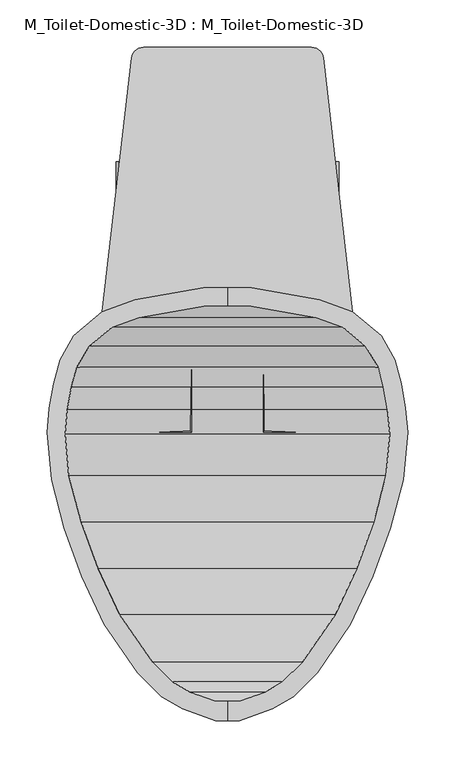
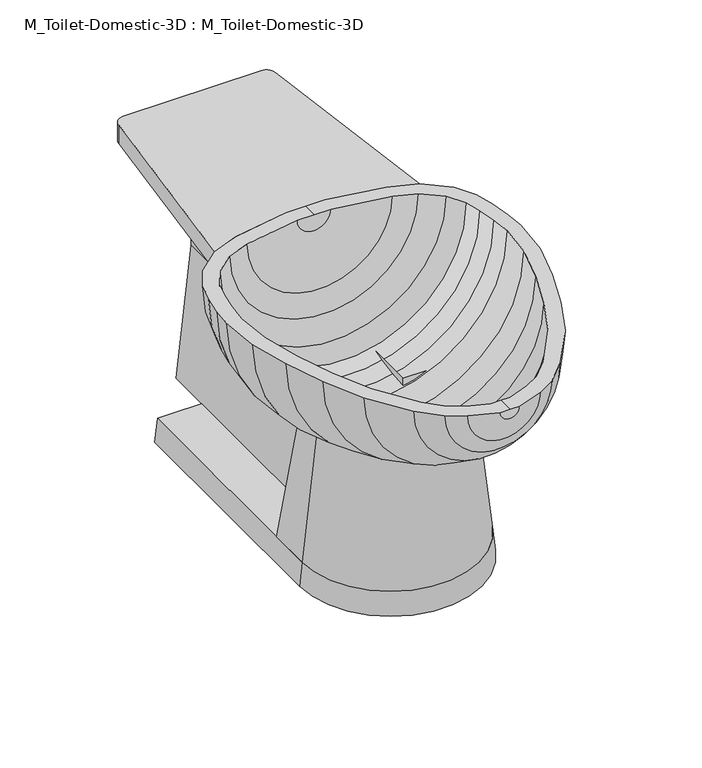
"""IFC4 building model written with IfcOpenShell, lengths in millimetres: flow terminal geometry, M_Toilet-Domestic-3D : M_Toilet-Domestic-3D."""

from ifc_helpers import new_model, si_unit, point, frame, frame_2d, origin, place, context, project, spatial, polyline, circle_curve, trimmed, segment, composite_curve, outline, extrude, source, transform, mapped, element, save
from ifc_brep_helpers import plane_surface, revolved_surface, advanced_brep


def m_toilet_domestic_3d_m_toilet_domestic_3d_ba6479b0(model_context):
    return source(origin(), model_context, "Body", "SolidModel", [
        advanced_brep(
        [(-25.4, 152.4, 361.95), (-97.4252791, 139.7, 361.95), (-132.3182423, 127.0, 361.95), (-162.5887836, 101.6, 361.95), (-176.9845865, 76.2, 361.95), (-183.790496, 50.8, 361.95), (-188.2862441, 25.3033453, 361.95), (-190.5, 0.0, 361.95), (-186.0724883, -50.6066907, 361.95), (-172.4088722, -101.6, 361.95), (-153.9191843, -152.4, 361.95), (-130.2307553, -203.2, 361.95), (-94.9900085, -254.0, 361.95), (-69.5900085, -279.4, 361.95), (-47.5929632, -292.1, 361.95), (-12.7, -304.8, 361.95), (0.0, -304.8, 361.95), (0.0, -284.592034, 361.95), (-12.5224565, -284.592034, 361.95), (-39.5113323, -274.7688865, 361.95), (-58.4178985, -263.8531754, 361.95), (-79.2146703, -243.0564036, 361.95), (-114.0255101, -192.8761202, 361.95), (-136.654021, -144.3491221, 361.95), (-154.575847, -95.1093097, 361.95), (-167.7238545, -46.0402777, 361.95), (-171.5645445, -2.1409906, 361.95), (-169.3087351, 23.6430284, 361.95), (-165.101298, 47.5045901, 361.95), (-159.5484355, 68.2281551, 361.95), (-146.1085923, 90.5605136, 361.95), (-121.9980886, 110.7916284, 361.95), (-94.1172813, 120.9394123, 361.95), (-22.0920022, 133.6394123, 361.95), (0.0, 133.6394123, 361.95), (0.0, 152.4, 361.95), (25.4, 152.4, 361.95), (22.0920022, 133.6394123, 361.95), (94.1172813, 120.9394123, 361.95), (121.9980886, 110.7916284, 361.95), (146.1085923, 90.5605136, 361.95), (159.5484355, 68.2281551, 361.95), (165.101298, 47.5045901, 361.95), (169.3087351, 23.6430284, 361.95), (171.5645445, -2.1409906, 361.95), (167.7238545, -46.0402777, 361.95), (154.575847, -95.1093097, 361.95), (136.654021, -144.3491221, 361.95), (114.0255101, -192.8761202, 361.95), (79.2146703, -243.0564036, 361.95), (58.4178985, -263.8531754, 361.95), (39.5113323, -274.7688865, 361.95), (12.5224565, -284.592034, 361.95), (12.7, -304.8, 361.95), (47.5929632, -292.1, 361.95), (69.5900085, -279.4, 361.95), (94.9900085, -254.0, 361.95), (130.2307553, -203.2, 361.95), (153.9191843, -152.4, 361.95), (172.4088722, -101.6, 361.95), (186.0724883, -50.6066907, 361.95), (190.5, 0.0, 361.95), (188.2862441, 25.3033453, 361.95), (183.790496, 50.8, 361.95), (176.9845865, 76.2, 361.95), (162.5887836, 101.6, 361.95), (132.3182423, 127.0, 361.95), (97.4252791, 139.7, 361.95)],
        [
            (0, 1),
            (1, 2),
            (2, 3),
            (3, 4),
            (4, 5),
            (5, 6),
            (6, 7),
            (7, 8),
            (8, 9),
            (9, 10),
            (10, 11),
            (11, 12),
            (12, 13),
            (13, 14),
            (14, 15),
            (15, 16),
            (16, 17),
            (17, 18),
            (18, 19),
            (19, 20),
            (20, 21),
            (21, 22),
            (22, 23),
            (23, 24),
            (24, 25),
            (25, 26),
            (26, 27),
            (27, 28),
            (28, 29),
            (29, 30),
            (30, 31),
            (31, 32),
            (32, 33),
            (33, 34),
            (34, 35),
            (35, 0),
            (36, 35),
            (34, 37),
            (37, 38),
            (38, 39),
            (39, 40),
            (40, 41),
            (41, 42),
            (42, 43),
            (43, 44),
            (44, 45),
            (45, 46),
            (46, 47),
            (47, 48),
            (48, 49),
            (49, 50),
            (50, 51),
            (51, 52),
            (52, 17),
            (16, 53),
            (53, 54),
            (54, 55),
            (55, 56),
            (56, 57),
            (57, 58),
            (58, 59),
            (59, 60),
            (60, 61),
            (61, 62),
            (62, 63),
            (63, 64),
            (64, 65),
            (65, 66),
            (66, 67),
            (67, 36),
            (67, 1, circle_curve(frame((0.0, 139.7, 361.95), z_axis=(0.0, 1.0, 0.0), x_axis=(-1.0, 0.0, 0.0)), 97.4252791)),
            (0, 36, circle_curve(frame((0.0, 152.4, 361.95), z_axis=(0.0, -1.0, 0.0), x_axis=(-1.0, 0.0, 0.0)), 25.4)),
            (66, 2, circle_curve(frame((0.0, 127.0, 361.95), z_axis=(0.0, 1.0, 0.0), x_axis=(-1.0, 0.0, 0.0)), 132.3182423)),
            (65, 3, circle_curve(frame((0.0, 101.6, 361.95), z_axis=(0.0, 1.0, 0.0), x_axis=(-1.0, 0.0, 0.0)), 162.5887836)),
            (64, 4, circle_curve(frame((0.0, 76.2, 361.95), z_axis=(0.0, 1.0, 0.0), x_axis=(-1.0, 0.0, 0.0)), 176.9845865)),
            (63, 5, circle_curve(frame((0.0, 50.8, 361.95), z_axis=(0.0, 1.0, 0.0), x_axis=(-1.0, 0.0, 0.0)), 183.790496)),
            (62, 6, circle_curve(frame((0.0, 25.3033453, 361.95), z_axis=(0.0, 1.0, 0.0), x_axis=(-1.0, 0.0, 0.0)), 188.2862441)),
            (61, 7, circle_curve(frame((0.0, 0.0, 361.95), z_axis=(0.0, 1.0, 0.0), x_axis=(-1.0, 0.0, 0.0)), 190.5)),
            (60, 8, circle_curve(frame((0.0, -50.6066907, 361.95), z_axis=(0.0, 1.0, 0.0), x_axis=(-1.0, 0.0, 0.0)), 186.0724883)),
            (59, 9, circle_curve(frame((0.0, -101.6, 361.95), z_axis=(0.0, 1.0, 0.0), x_axis=(-1.0, 0.0, 0.0)), 172.4088722)),
            (58, 10, circle_curve(frame((0.0, -152.4, 361.95), z_axis=(0.0, 1.0, 0.0), x_axis=(-1.0, 0.0, 0.0)), 153.9191843)),
            (57, 11, circle_curve(frame((0.0, -203.2, 361.95), z_axis=(0.0, 1.0, 0.0), x_axis=(-1.0, 0.0, 0.0)), 130.2307553)),
            (56, 12, circle_curve(frame((0.0, -254.0, 361.95), z_axis=(0.0, 1.0, 0.0), x_axis=(-1.0, 0.0, 0.0)), 94.9900085)),
            (55, 13, circle_curve(frame((0.0, -279.4, 361.95), z_axis=(0.0, 1.0, 0.0), x_axis=(-1.0, 0.0, 0.0)), 69.5900085)),
            (54, 14, circle_curve(frame((0.0, -292.1, 361.95), z_axis=(0.0, 1.0, 0.0), x_axis=(-1.0, 0.0, 0.0)), 47.5929632)),
            (53, 15, circle_curve(frame((0.0, -304.8, 361.95), z_axis=(0.0, 1.0, 0.0), x_axis=(-1.0, 0.0, 0.0)), 12.7)),
            (52, 18, circle_curve(frame((0.0, -284.592034, 361.95), z_axis=(0.0, 1.0, 0.0), x_axis=(-1.0, 0.0, 0.0)), 12.5224565)),
            (51, 19, circle_curve(frame((0.0, -274.7688865, 361.95), z_axis=(0.0, 1.0, 0.0), x_axis=(-1.0, 0.0, 0.0)), 39.5113323)),
            (50, 20, circle_curve(frame((0.0, -263.8531754, 361.95), z_axis=(0.0, 1.0, 0.0), x_axis=(-1.0, 0.0, 0.0)), 58.4178985)),
            (49, 21, circle_curve(frame((0.0, -243.0564036, 361.95), z_axis=(0.0, 1.0, 0.0), x_axis=(-1.0, 0.0, 0.0)), 79.2146703)),
            (48, 22, circle_curve(frame((0.0, -192.8761202, 361.95), z_axis=(0.0, 1.0, 0.0), x_axis=(-1.0, 0.0, 0.0)), 114.0255101)),
            (47, 23, circle_curve(frame((0.0, -144.3491221, 361.95), z_axis=(0.0, 1.0, 0.0), x_axis=(-1.0, 0.0, 0.0)), 136.654021)),
            (46, 24, circle_curve(frame((0.0, -95.1093097, 361.95), z_axis=(0.0, 1.0, 0.0), x_axis=(-1.0, 0.0, 0.0)), 154.575847)),
            (45, 25, circle_curve(frame((0.0, -46.0402777, 361.95), z_axis=(0.0, 1.0, 0.0), x_axis=(-1.0, 0.0, 0.0)), 167.7238545)),
            (44, 26, circle_curve(frame((0.0, -2.1409906, 361.95), z_axis=(0.0, 1.0, 0.0), x_axis=(-1.0, 0.0, 0.0)), 171.5645445)),
            (43, 27, circle_curve(frame((0.0, 23.6430284, 361.95), z_axis=(0.0, 1.0, 0.0), x_axis=(-1.0, 0.0, 0.0)), 169.3087351)),
            (42, 28, circle_curve(frame((0.0, 47.5045901, 361.95), z_axis=(0.0, 1.0, 0.0), x_axis=(-1.0, 0.0, 0.0)), 165.101298)),
            (41, 29, circle_curve(frame((0.0, 68.2281551, 361.95), z_axis=(0.0, 1.0, 0.0), x_axis=(-1.0, 0.0, 0.0)), 159.5484355)),
            (40, 30, circle_curve(frame((0.0, 90.5605136, 361.95), z_axis=(0.0, 1.0, 0.0), x_axis=(-1.0, 0.0, 0.0)), 146.1085923)),
            (39, 31, circle_curve(frame((0.0, 110.7916284, 361.95), z_axis=(0.0, 1.0, 0.0), x_axis=(-1.0, 0.0, 0.0)), 121.9980886)),
            (38, 32, circle_curve(frame((0.0, 120.9394123, 361.95), z_axis=(0.0, 1.0, 0.0), x_axis=(-1.0, 0.0, 0.0)), 94.1172813)),
            (37, 33, circle_curve(frame((0.0, 133.6394123, 361.95), z_axis=(0.0, 1.0, 0.0), x_axis=(-1.0, 0.0, 0.0)), 22.0920022)),
        ],
        [
            plane_surface(frame((0.0, 175.1599017, 361.95), z_axis=(0.0, 0.0, 1.0), x_axis=(-1.0, 0.0, 0.0))),
            plane_surface(frame((0.0, 175.1599017, 361.95), z_axis=(0.0, 0.0, 1.0), x_axis=(1.0, 0.0, 0.0))),
            revolved_surface(polyline([(-25.4, 152.4, 361.95), (-97.4252791, 139.7, 361.95)]), (0.0, 175.1599017, 361.95), (0.0, -1.0, 0.0)),
            revolved_surface(polyline([(-97.4252791, 139.7, 361.95), (-132.3182423, 127.0, 361.95)]), (0.0, 175.1599017, 361.95), (0.0, -1.0, 0.0)),
            revolved_surface(polyline([(-132.3182423, 127.0, 361.95), (-162.5887836, 101.6, 361.95)]), (0.0, 175.1599017, 361.95), (0.0, -1.0, 0.0)),
            revolved_surface(polyline([(-162.5887836, 101.6, 361.95), (-176.9845865, 76.2, 361.95)]), (0.0, 175.1599017, 361.95), (0.0, -1.0, 0.0)),
            revolved_surface(polyline([(-176.9845865, 76.2, 361.95), (-183.790496, 50.8, 361.95)]), (0.0, 175.1599017, 361.95), (0.0, -1.0, 0.0)),
            revolved_surface(polyline([(-183.790496, 50.8, 361.95), (-188.2862441, 25.3033453, 361.95)]), (0.0, 175.1599017, 361.95), (0.0, -1.0, 0.0)),
            revolved_surface(polyline([(-188.2862441, 25.3033453, 361.95), (-190.5, 0.0, 361.95)]), (0.0, 175.1599017, 361.95), (0.0, -1.0, 0.0)),
            revolved_surface(polyline([(-190.5, 0.0, 361.95), (-186.0724883, -50.6066907, 361.95)]), (0.0, 175.1599017, 361.95), (0.0, -1.0, 0.0)),
            revolved_surface(polyline([(-186.0724883, -50.6066907, 361.95), (-172.4088722, -101.6, 361.95)]), (0.0, 175.1599017, 361.95), (0.0, -1.0, 0.0)),
            revolved_surface(polyline([(-172.4088722, -101.6, 361.95), (-153.9191843, -152.4, 361.95)]), (0.0, 175.1599017, 361.95), (0.0, -1.0, 0.0)),
            revolved_surface(polyline([(-153.9191843, -152.4, 361.95), (-130.2307553, -203.2, 361.95)]), (0.0, 175.1599017, 361.95), (0.0, -1.0, 0.0)),
            revolved_surface(polyline([(-130.2307553, -203.2, 361.95), (-94.9900085, -254.0, 361.95)]), (0.0, 175.1599017, 361.95), (0.0, -1.0, 0.0)),
            revolved_surface(polyline([(-94.9900085, -254.0, 361.95), (-69.5900085, -279.4, 361.95)]), (0.0, 175.1599017, 361.95), (0.0, -1.0, 0.0)),
            revolved_surface(polyline([(-69.5900085, -279.4, 361.95), (-47.5929632, -292.1, 361.95)]), (0.0, 175.1599017, 361.95), (0.0, -1.0, 0.0)),
            revolved_surface(polyline([(-47.5929632, -292.1, 361.95), (-12.7, -304.8, 361.95)]), (0.0, 175.1599017, 361.95), (0.0, -1.0, 0.0)),
            plane_surface(frame((0.0, -304.8, 361.95), z_axis=(0.0, -1.0, 0.0), x_axis=(-1.0, 0.0, 0.0))),
            plane_surface(frame((0.0, -284.592034, 361.95), z_axis=(0.0, 1.0, 0.0), x_axis=(-1.0, 0.0, 0.0))),
            revolved_surface(polyline([(-12.5224565, -284.592034, 361.95), (-39.5113323, -274.7688865, 361.95)]), (0.0, 175.1599017, 361.95), (0.0, -1.0, 0.0)),
            revolved_surface(polyline([(-39.5113323, -274.7688865, 361.95), (-58.4178985, -263.8531754, 361.95)]), (0.0, 175.1599017, 361.95), (0.0, -1.0, 0.0)),
            revolved_surface(polyline([(-58.4178985, -263.8531754, 361.95), (-79.2146703, -243.0564036, 361.95)]), (0.0, 175.1599017, 361.95), (0.0, -1.0, 0.0)),
            revolved_surface(polyline([(-79.2146703, -243.0564036, 361.95), (-114.0255101, -192.8761202, 361.95)]), (0.0, 175.1599017, 361.95), (0.0, -1.0, 0.0)),
            revolved_surface(polyline([(-114.0255101, -192.8761202, 361.95), (-136.654021, -144.3491221, 361.95)]), (0.0, 175.1599017, 361.95), (0.0, -1.0, 0.0)),
            revolved_surface(polyline([(-136.654021, -144.3491221, 361.95), (-154.575847, -95.1093097, 361.95)]), (0.0, 175.1599017, 361.95), (0.0, -1.0, 0.0)),
            revolved_surface(polyline([(-154.575847, -95.1093097, 361.95), (-167.7238545, -46.0402777, 361.95)]), (0.0, 175.1599017, 361.95), (0.0, -1.0, 0.0)),
            revolved_surface(polyline([(-167.7238545, -46.0402777, 361.95), (-171.5645445, -2.1409906, 361.95)]), (0.0, 175.1599017, 361.95), (0.0, -1.0, 0.0)),
            revolved_surface(polyline([(-171.5645445, -2.1409906, 361.95), (-169.3087351, 23.6430284, 361.95)]), (0.0, 175.1599017, 361.95), (0.0, -1.0, 0.0)),
            revolved_surface(polyline([(-169.3087351, 23.6430284, 361.95), (-165.101298, 47.5045901, 361.95)]), (0.0, 175.1599017, 361.95), (0.0, -1.0, 0.0)),
            revolved_surface(polyline([(-165.101298, 47.5045901, 361.95), (-159.5484355, 68.2281551, 361.95)]), (0.0, 175.1599017, 361.95), (0.0, -1.0, 0.0)),
            revolved_surface(polyline([(-159.5484355, 68.2281551, 361.95), (-146.1085923, 90.5605136, 361.95)]), (0.0, 175.1599017, 361.95), (0.0, -1.0, 0.0)),
            revolved_surface(polyline([(-146.1085923, 90.5605136, 361.95), (-121.9980886, 110.7916284, 361.95)]), (0.0, 175.1599017, 361.95), (0.0, -1.0, 0.0)),
            revolved_surface(polyline([(-121.9980886, 110.7916284, 361.95), (-94.1172813, 120.9394123, 361.95)]), (0.0, 175.1599017, 361.95), (0.0, -1.0, 0.0)),
            revolved_surface(polyline([(-94.1172813, 120.9394123, 361.95), (-22.0920022, 133.6394123, 361.95)]), (0.0, 175.1599017, 361.95), (0.0, -1.0, 0.0)),
            plane_surface(frame((0.0, 133.6394123, 361.95), z_axis=(0.0, -1.0, 0.0), x_axis=(-1.0, 0.0, 0.0))),
            plane_surface(frame((0.0, 152.4, 361.95), z_axis=(0.0, 1.0, 0.0), x_axis=(-1.0, 0.0, 0.0))),
        ],
        [
            (0, [[1, 2, 3, 4, 5, 6, 7, 8, 9, 10, 11, 12, 13, 14, 15, 16, 17, 18, 19, 20, 21, 22, 23, 24, 25, 26, 27, 28, 29, 30, 31, 32, 33, 34, 35, 36]]),
            (1, [[37, -35, 38, 39, 40, 41, 42, 43, 44, 45, 46, 47, 48, 49, 50, 51, 52, 53, 54, -17, 55, 56, 57, 58, 59, 60, 61, 62, 63, 64, 65, 66, 67, 68, 69, 70]]),
            (2, [[71, -1, 72, -70]]),
            (3, [[73, -2, -71, -69]]),
            (4, [[74, -3, -73, -68]]),
            (5, [[75, -4, -74, -67]]),
            (6, [[76, -5, -75, -66]]),
            (7, [[77, -6, -76, -65]]),
            (8, [[78, -7, -77, -64]]),
            (9, [[79, -8, -78, -63]]),
            (10, [[80, -9, -79, -62]]),
            (11, [[81, -10, -80, -61]]),
            (12, [[82, -11, -81, -60]]),
            (13, [[83, -12, -82, -59]]),
            (14, [[84, -13, -83, -58]]),
            (15, [[85, -14, -84, -57]]),
            (16, [[86, -15, -85, -56]]),
            (17, [[-16, -86, -55]]),
            (18, [[87, -18, -54]]),
            (19, [[88, -19, -87, -53]]),
            (20, [[89, -20, -88, -52]]),
            (21, [[90, -21, -89, -51]]),
            (22, [[91, -22, -90, -50]]),
            (23, [[92, -23, -91, -49]]),
            (24, [[93, -24, -92, -48]]),
            (25, [[94, -25, -93, -47]]),
            (26, [[95, -26, -94, -46]]),
            (27, [[96, -27, -95, -45]]),
            (28, [[97, -28, -96, -44]]),
            (29, [[98, -29, -97, -43]]),
            (30, [[99, -30, -98, -42]]),
            (31, [[100, -31, -99, -41]]),
            (32, [[101, -32, -100, -40]]),
            (33, [[102, -33, -101, -39]]),
            (34, [[-34, -102, -38]]),
            (35, [[-72, -36, -37]]),
        ],
    ),
        advanced_brep(
        [(-57.15, 342.9, 31.75), (-38.1, 342.9, 206.375), (-38.1, 342.9, 31.75), (-57.15, 19.05, 31.75), (-38.1, 0.0, 206.375), (-38.1, 0.0, 31.75), (-114.3, 19.05, 31.75), (-95.25, 0.0, 206.375), (-95.25, 0.0, 31.75), (-114.3, -38.1, 31.75), (-95.25, -38.1, 206.375), (-95.25, -38.1, 31.75), (95.25, -38.1, 206.375), (114.3, -38.1, 31.75), (95.25, -38.1, 31.75), (114.3, 19.05, 31.75), (95.25, 0.0, 206.375), (95.25, 0.0, 31.75), (57.15, 19.05, 31.75), (38.1, 0.0, 206.375), (38.1, 0.0, 31.75), (57.15, 342.9, 31.75), (38.1, 342.9, 31.75), (38.1, 342.9, 206.375)],
        [
            (0, 1),
            (1, 2),
            (2, 0),
            (0, 3),
            (3, 4),
            (4, 1),
            (4, 5),
            (5, 2),
            (5, 3),
            (3, 6),
            (6, 7),
            (7, 4),
            (7, 8),
            (8, 5),
            (8, 6),
            (6, 9),
            (9, 10),
            (10, 7),
            (10, 11),
            (11, 8),
            (11, 9),
            (12, 10, circle_curve(frame((0.0, -38.1, 206.375), z_axis=(0.0, 0.0, -1.0), x_axis=(-1.0, 0.0, 0.0)), 95.25)),
            (9, 13, circle_curve(frame((0.0, -38.1, 31.75), z_axis=(0.0, 0.0, 1.0), x_axis=(-1.0, 0.0, 0.0)), 114.3)),
            (13, 12),
            (14, 11, circle_curve(frame((0.0, -38.1, 31.75), z_axis=(0.0, 0.0, -1.0), x_axis=(-1.0, 0.0, 0.0)), 95.25)),
            (12, 14),
            (14, 13),
            (13, 15),
            (15, 16),
            (16, 12),
            (16, 17),
            (17, 14),
            (17, 15),
            (15, 18),
            (18, 19),
            (19, 16),
            (19, 20),
            (20, 17),
            (20, 18),
            (21, 22),
            (22, 23),
            (23, 21),
            (18, 21),
            (23, 19),
            (22, 20),
        ],
        [
            plane_surface(frame((-244.475, 342.9, 0.0), z_axis=(0.0, 1.0, 0.0), x_axis=(0.0, 0.0, -1.0))),
            plane_surface(frame((-57.15, 342.9, 31.75), z_axis=(-0.9941021766079944, 0.0, 0.10844751017542063), x_axis=(0.0, -1.0, 0.0))),
            plane_surface(frame((-38.1, 342.9, 206.375), z_axis=(1.0, 0.0, 0.0), x_axis=(0.0, -1.0, 0.0))),
            plane_surface(frame((-38.1, 342.9, 31.75), z_axis=(0.0, 0.0, -1.0), x_axis=(0.0, -1.0, 0.0))),
            plane_surface(frame((-57.15, 19.05, 31.75), z_axis=(0.0, 0.9941021766079944, 0.10844751017542063), x_axis=(-1.0, 0.0, 0.0))),
            plane_surface(frame((-38.1, 0.0, 206.375), z_axis=(0.0, -1.0, 0.0), x_axis=(-1.0, 0.0, 0.0))),
            plane_surface(frame((-38.1, 0.0, 31.75), z_axis=(0.0, 0.0, -1.0), x_axis=(-1.0, 0.0, 0.0))),
            plane_surface(frame((-114.3, 19.05, 31.75), z_axis=(-0.9941021766079944, 0.0, 0.10844751017542063), x_axis=(0.0, -1.0, 0.0))),
            plane_surface(frame((-95.25, 0.0, 206.375), z_axis=(1.0, 0.0, 0.0), x_axis=(0.0, -1.0, 0.0))),
            plane_surface(frame((-95.25, 0.0, 31.75), z_axis=(0.0, 0.0, -1.0), x_axis=(0.0, -1.0, 0.0))),
            revolved_surface(polyline([(-114.3, -38.1, 31.75), (-95.25, -38.1, 206.375)]), (0.0, -38.1, 0.0), (0.0, 0.0, 1.0)),
            revolved_surface(polyline([(-95.25, -38.1, 206.375), (-95.25, -38.1, 31.75)]), (0.0, -38.1, 0.0), (0.0, 0.0, 1.0)),
            plane_surface(frame((0.0, -38.1, 31.75), z_axis=(0.0, 0.0, -1.0), x_axis=(-1.0, 0.0, 0.0))),
            plane_surface(frame((114.3, -38.1, 31.75), z_axis=(0.9941021766079944, 0.0, 0.10844751017542063), x_axis=(0.0, 1.0, 0.0))),
            plane_surface(frame((95.25, -38.1, 206.375), z_axis=(-1.0, 0.0, 0.0), x_axis=(0.0, 1.0, 0.0))),
            plane_surface(frame((95.25, -38.1, 31.75), z_axis=(0.0, 0.0, -1.0), x_axis=(0.0, 1.0, 0.0))),
            plane_surface(frame((114.3, 19.05, 31.75), z_axis=(0.0, 0.9941021766079944, 0.10844751017542063), x_axis=(-1.0, 0.0, 0.0))),
            plane_surface(frame((95.25, 0.0, 206.375), z_axis=(0.0, -1.0, 0.0), x_axis=(-1.0, 0.0, 0.0))),
            plane_surface(frame((95.25, 0.0, 31.75), z_axis=(0.0, 0.0, -1.0), x_axis=(-1.0, 0.0, 0.0))),
            plane_surface(frame((-168.275, 342.9, 0.0), z_axis=(0.0, 1.0, 0.0), x_axis=(0.0, 0.0, 1.0))),
            plane_surface(frame((57.15, 19.05, 31.75), z_axis=(0.9941021766079944, 0.0, 0.10844751017542063), x_axis=(0.0, 1.0, 0.0))),
            plane_surface(frame((38.1, 0.0, 206.375), z_axis=(-1.0, 0.0, 0.0), x_axis=(0.0, 1.0, 0.0))),
            plane_surface(frame((38.1, 0.0, 31.75), z_axis=(0.0, 0.0, -1.0), x_axis=(0.0, 1.0, 0.0))),
        ],
        [
            (0, [[1, 2, 3]]),
            (1, [[-1, 4, 5, 6]]),
            (2, [[-2, -6, 7, 8]]),
            (3, [[-3, -8, 9, -4]]),
            (4, [[-5, 10, 11, 12]]),
            (5, [[-7, -12, 13, 14]]),
            (6, [[-9, -14, 15, -10]]),
            (7, [[-11, 16, 17, 18]]),
            (8, [[-13, -18, 19, 20]]),
            (9, [[-15, -20, 21, -16]]),
            (10, [[22, -17, 23, 24]]),
            (11, [[25, -19, -22, 26]]),
            (12, [[-23, -21, -25, 27]]),
            (13, [[-24, 28, 29, 30]]),
            (14, [[-26, -30, 31, 32]]),
            (15, [[-27, -32, 33, -28]]),
            (16, [[-29, 34, 35, 36]]),
            (17, [[-31, -36, 37, 38]]),
            (18, [[-33, -38, 39, -34]]),
            (19, [[40, 41, 42]]),
            (20, [[-35, 43, -42, 44]]),
            (21, [[-37, -44, -41, 45]]),
            (22, [[-39, -45, -40, -43]]),
        ],
    ),
        advanced_brep(
        [(-117.7636364, 285.75, 0.0), (-114.3, 285.75, 31.75), (-38.1, 285.75, 31.75), (-38.1, 285.75, 0.0), (-117.7636364, -38.0999951, 0.0), (-114.3, -38.0999951, 31.75), (-38.1, -38.0999951, 31.75), (-38.1, -38.0999951, 0.0), (114.2999707, -38.0999951, 31.75), (117.7636071, -38.0999951, 0.0), (38.0999707, -38.0999951, 31.75), (38.0999707, -38.0999951, 0.0), (117.7636071, 285.6681634, 0.0), (38.0999707, 285.6681634, 0.0), (38.0999707, 285.6681634, 31.75), (114.2999707, 285.6681634, 31.75)],
        [
            (0, 1),
            (1, 2),
            (2, 3),
            (3, 0),
            (0, 4),
            (4, 5),
            (5, 1),
            (5, 6),
            (6, 2),
            (6, 7),
            (7, 3),
            (7, 4),
            (8, 5, circle_curve(frame((-1.46e-05, -38.0999951, 31.75), z_axis=(0.0, 0.0, -1.0), x_axis=(-1.0, 0.0, 0.0)), 114.2999854)),
            (4, 9, circle_curve(frame((-1.46e-05, -38.0999951, 0.0), z_axis=(0.0, 0.0, 1.0), x_axis=(-1.0, 0.0, 0.0)), 117.7636217)),
            (9, 8),
            (10, 6, circle_curve(frame((-1.46e-05, -38.0999951, 31.75), z_axis=(0.0, 0.0, -1.0), x_axis=(-1.0, 0.0, 0.0)), 38.0999854)),
            (8, 10),
            (11, 7, circle_curve(frame((-1.46e-05, -38.0999951, 0.0), z_axis=(0.0, 0.0, -1.0), x_axis=(-1.0, 0.0, 0.0)), 38.0999854)),
            (10, 11),
            (11, 9),
            (12, 13),
            (13, 14),
            (14, 15),
            (15, 12),
            (9, 12),
            (15, 8),
            (14, 10),
            (13, 11),
        ],
        [
            plane_surface(frame((-196.85, 285.75, 0.0), z_axis=(0.0, 1.0, 0.0), x_axis=(0.0, 0.0, -1.0))),
            plane_surface(frame((-117.7636364, 285.75, 0.0), z_axis=(-0.9941021766079929, 0.0, 0.10844751017543448), x_axis=(0.0, -1.0, 0.0))),
            plane_surface(frame((-114.3, 285.75, 31.75), z_axis=(0.0, 0.0, 1.0), x_axis=(0.0, -1.0, 0.0))),
            plane_surface(frame((-38.1, 285.75, 31.75), z_axis=(1.0, 0.0, 0.0), x_axis=(0.0, -1.0, 0.0))),
            plane_surface(frame((-38.1, 285.75, 0.0), z_axis=(0.0, 0.0, -1.0), x_axis=(0.0, -1.0, 0.0))),
            revolved_surface(polyline([(-117.7636364, -38.0999951, 0.0), (-114.3, -38.0999951, 31.75)]), (-1.46e-05, -38.0999951, 0.0), (0.0, 0.0, 1.0)),
            plane_surface(frame((-1.46e-05, -38.0999951, 31.75), z_axis=(0.0, 0.0, 1.0), x_axis=(-1.0, 0.0, 0.0))),
            revolved_surface(polyline([(-38.1, -38.0999951, 31.75), (-38.1, -38.0999951, 0.0)]), (-1.46e-05, -38.0999951, 0.0), (0.0, 0.0, 1.0)),
            plane_surface(frame((-1.46e-05, -38.0999951, 0.0), z_axis=(0.0, 0.0, -1.0), x_axis=(-1.0, 0.0, 0.0))),
            plane_surface(frame((31.7499707, 285.6681634, 0.0), z_axis=(0.0, 1.0, 0.0), x_axis=(0.0, 0.0, 1.0))),
            plane_surface(frame((117.7636071, -38.0999951, 0.0), z_axis=(0.9941021766079929, 0.0, 0.10844751017543448), x_axis=(0.0, 1.0, 0.0))),
            plane_surface(frame((114.2999707, -38.0999951, 31.75), z_axis=(0.0, 0.0, 1.0), x_axis=(0.0, 1.0, 0.0))),
            plane_surface(frame((38.0999707, -38.0999951, 31.75), z_axis=(-1.0, 0.0, 0.0), x_axis=(0.0, 1.0, 0.0))),
            plane_surface(frame((38.0999707, -38.0999951, 0.0), z_axis=(0.0, 0.0, -1.0), x_axis=(0.0, 1.0, 0.0))),
        ],
        [
            (0, [[1, 2, 3, 4]]),
            (1, [[-1, 5, 6, 7]]),
            (2, [[-2, -7, 8, 9]]),
            (3, [[-3, -9, 10, 11]]),
            (4, [[-4, -11, 12, -5]]),
            (5, [[13, -6, 14, 15]]),
            (6, [[16, -8, -13, 17]]),
            (7, [[18, -10, -16, 19]]),
            (8, [[-14, -12, -18, 20]]),
            (9, [[21, 22, 23, 24]]),
            (10, [[-15, 25, -24, 26]]),
            (11, [[-17, -26, -23, 27]]),
            (12, [[-19, -27, -22, 28]]),
            (13, [[-20, -28, -21, -25]]),
        ],
    ),
        extrude(outline(polyline([(139.7, 264.5247209), (152.4, 336.55), (342.9, 336.55), (342.9, 206.375), (107.4852632, 206.375), (127.0, 229.6317577), (139.7, 264.5247209)])), frame((-38.1, 0.0, 0.0), z_axis=(1.0, 0.0, 0.0), x_axis=(0.0, 1.0, 0.0)), (0.0, 0.0, 1.0), 76.2),
        extrude(outline(composite_curve([segment(polyline([(-25.4, 152.4), (-97.4252791, 139.7), (-132.3182423, 127.0), (-101.4824733, 395.1508638)]), True, "CONTINUOUS"), segment(trimmed(circle_curve(frame_2d((-88.8656197, 393.7)), 12.7), [point((-101.4824733, 395.1508638))], [point((-88.8656197, 406.4))], False, "CARTESIAN"), True, "CONTINUOUS"), segment(polyline([(-88.8656197, 406.4), (88.8656197, 406.4)]), True, "CONTINUOUS"), segment(trimmed(circle_curve(frame_2d((88.8656197, 393.7)), 12.7), [point((88.8656197, 406.4))], [point((101.4824733, 395.1508638))], False, "CARTESIAN"), True, "CONTINUOUS"), segment(polyline([(101.4824733, 395.1508638), (132.3182423, 127.0), (97.4252791, 139.7), (25.4, 152.4), (0.0, 152.4), (-25.4, 152.4)]), True, "CONTINUOUS")], self_intersect=False)), frame((0.0, 0.0, 336.55), z_axis=(0.0, 0.0, 1.0), x_axis=(1.0, 0.0, 0.0)), (0.0, 0.0, 1.0), 25.4),
    ])


if __name__ == "__main__":
    model = new_model("IFC4")
    model_context = context("Model", 3, world=origin())
    ifc_project = project(units=[si_unit("LENGTHUNIT", "METRE", prefix="MILLI")], contexts=[model_context])
    site = spatial("IfcSite", under=ifc_project)
    building = spatial("IfcBuilding", under=site)
    placement = place(None, origin())
    m_toilet_domestic_3d_m_toilet_domestic_3d_shape = m_toilet_domestic_3d_m_toilet_domestic_3d_ba6479b0(model_context)
    element("IfcFlowTerminal", 1, ObjectType="M_Toilet-Domestic-3D : M_Toilet-Domestic-3D", at=placement, inside=building, context=model_context, shape_type="MappedRepresentation", body=[
        mapped(m_toilet_domestic_3d_m_toilet_domestic_3d_shape, transform((0.0, 0.0, 0.0), x_axis=(1.0, 0.0, 0.0), y_axis=(0.0, 1.0, 0.0), z_axis=(0.0, 0.0, 1.0))),
    ])
    save(model, "model.ifc")

# Revit data of these elements
# Type "M_Toilet-Domestic-3D : M_Toilet-Domestic-3D"
#   Bowl/Basin Material = Porcelain, Linen
#   Seat Material = Laminate, Linen, Matte
#   Default Elevation = 0
# Element 1 (IfcFlowTerminal, "M_Toilet-Domestic-3D : M_Toilet-Domestic-3D")
#   Materials on its faces: "Porcelain, Linen", "Laminate, Linen, Matte"
# Materials
#   "Porcelain, Linen": class "Ceramic", colour RGB 249 239 230, transparency 0, Description = "Porcelain, linen", Cost = 0
#   "Laminate, Linen, Matte": class "Plastic", colour RGB 249 239 230, transparency 0, Description = "Plastic Laminate - Linen, Matte", Cost = 0
